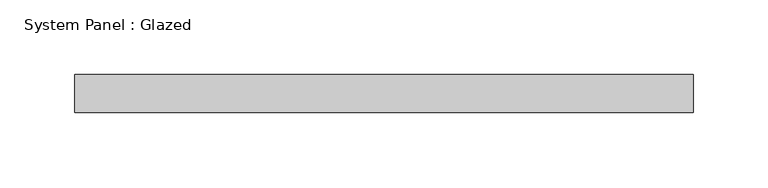
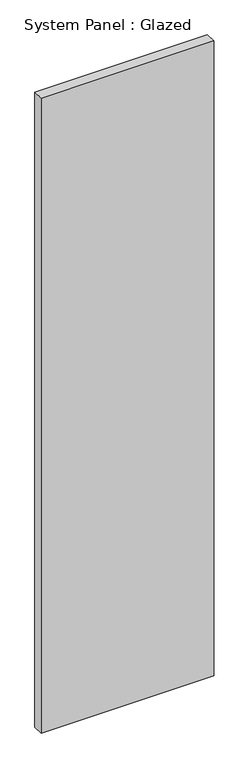
"""IFC4 building model written with IfcOpenShell, lengths in millimetres: plate geometry, System Panel : Glazed."""

from ifc_helpers import new_model, si_unit, origin, origin_with_axes, place, context, project, spatial, polyline, outline, extrude, source, transform, mapped, element, save


def system_panel_glazed_02abb1c2(model_context):
    return source(origin(), model_context, "Body", "SweptSolid", [
        extrude(outline(polyline([(206.375, 19.05), (-206.375, 19.05), (-206.375, 44.45), (206.375, 44.45), (206.375, 19.05)])), origin_with_axes(), (0.0, 0.0, 1.0), 1605.6965064),
    ])


if __name__ == "__main__":
    model = new_model("IFC4")
    model_context = context("Model", 3, world=origin())
    ifc_project = project(units=[si_unit("LENGTHUNIT", "METRE", prefix="MILLI")], contexts=[model_context])
    site = spatial("IfcSite", under=ifc_project)
    building = spatial("IfcBuilding", under=site)
    placement = place(None, origin())
    system_panel_glazed_shape = system_panel_glazed_02abb1c2(model_context)
    element("IfcPlate", 1, ObjectType="System Panel : Glazed", at=placement, inside=building, context=model_context, shape_type="MappedRepresentation", body=[
        mapped(system_panel_glazed_shape, transform((0.0, 0.0, 0.0), x_axis=(1.0, 0.0, 0.0), y_axis=(0.0, 1.0, 0.0), z_axis=(0.0, 0.0, 1.0))),
    ])
    save(model, "model.ifc")

# Revit data of these elements
# Type "System Panel : Glazed"
#   Construction Type Id = "GSP4R"
#   Analytic Construction = "1/8 in Pilkington single glazing"
#   Visual Light Transmittance = 0.9
#   Solar Heat Gain Coefficient = 0.86
#   Heat Transfer Coefficient (U) = 1.18115 BTU/(h·ft²·°F)
#   Define Thermal Properties by = 1
# Element 1 (IfcPlate, "System Panel : Glazed")
#   Materials on its faces: "Glass"
# Materials
#   "Glass": class "Glass", colour RGB 0 128 192, transparency 0.75, Description = "Soda Lime Glass", Cost = 0
